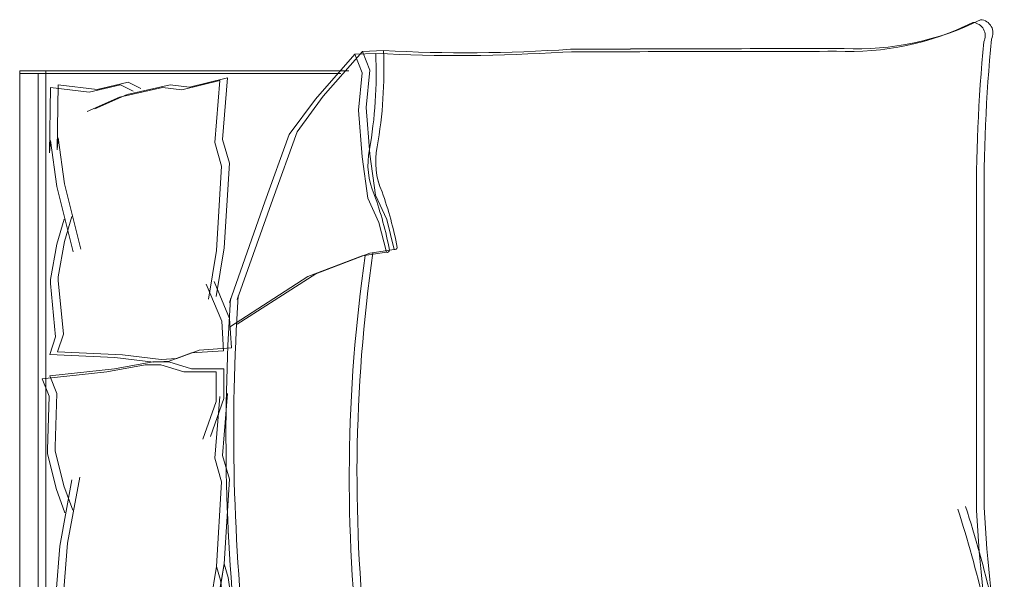
# Model space of a CAD drawing. Units: inches. Extents: x 1885 to 2748, y 783 to 2421.
# Tile 35 of 117: x 2014 to 2095, y 1443 to 1490. Entities that reach past the tile are written whole.
import ezdxf

# ---------------------------------------------------------------- set-up
doc = ezdxf.new("R2010")
doc.units = ezdxf.units.IN
doc.layers.add('A-FURN', color=8, linetype='Continuous', lineweight=13)

# ---------------------------------------------------------------- blocks, each defined once
blk = doc.blocks.new('BED-DOUBLE')
for p, q in [((28.389, 53.095), (25.139, 49.389)), ((28.389, 53.094), (25.139, 49.389)), ((30.133, 53.174), (28.389, 53.095, 3.871)), ((30.133, 53.174), (28.389, 53.094, 3.871)), ((29.008, 51.558), (28.389, 53.095)), ((29.008, 51.557), (28.389, 53.094)), ((27.749, 52.866), (24.499, 49.161)), ((27.75, 52.866), (24.499, 49.161)), ((29.494, 52.946), (27.749, 52.866, 3.871)), ((28.369, 51.329), (27.749, 52.866)), ((29.494, 52.945), (27.75, 52.866, 3.871)), ((28.369, 51.329), (27.75, 52.866)), ((0.004, 51.493), (0.643, 51.492)), ((0.004, 3.474), (0.004, 51.493)), ((0.643, 51.493), (27.253, 51.493)), ((0.643, 51.492), (27.253, 51.492)), ((2.177, 3.702), (2.177, 51.493)), ((2.177, 3.702), (2.177, 51.492)), ((28.698, 48.46), (29.008, 51.558)), ((28.698, 48.46), (29.008, 51.557)), ((0.004, 51.264), (26.614, 51.264)), ((0.004, 51.264), (26.614, 51.264)), ((1.537, 3.474), (1.537, 51.264)), ((1.537, 3.474), (1.537, 51.264)), ((16.576, 50.697), (13.438, 49.922)), ((16.576, 50.697), (13.438, 49.921)), ((17.216, 50.925), (14.077, 50.15)), ((17.216, 50.925), (14.077, 50.15)), ((16.173, 45.565), (16.576, 50.697)), ((16.173, 45.565), (16.576, 50.697)), ((16.812, 45.794), (17.216, 50.925)), ((16.812, 45.793), (17.216, 50.925)), ((28.059, 48.232), (28.369, 51.329)), ((28.059, 48.231), (28.369, 51.329)), ((2.561, 50.111), (2.464, 44.708)), ((2.561, 50.11), (2.464, 44.708)), ((2.561, 50.111), (5.771, 49.732)), ((2.561, 50.11), (5.771, 49.732)), ((3.2, 50.339), (3.103, 44.937)), ((3.2, 50.339), (3.103, 44.936)), ((3.2, 50.339), (6.411, 49.96)), ((3.2, 50.339), (6.411, 49.96)), ((5.771, 49.732), (8.342, 50.327)), ((5.771, 49.732), (8.342, 50.327)), ((6.411, 49.96), (8.981, 50.556)), ((6.411, 49.96), (8.981, 50.555)), ((11.832, 50.111), (8.261, 49.308)), ((11.832, 50.111), (8.261, 49.308)), ((8.342, 50.327), (9.388, 49.813)), ((8.342, 50.327), (9.388, 49.813)), ((12.472, 50.339), (8.9, 49.537)), ((12.472, 50.339), (8.9, 49.536)), ((8.981, 50.556), (10.027, 50.042)), ((8.981, 50.555), (10.027, 50.041)), ((13.438, 49.922), (11.832, 50.111)), ((13.438, 49.921), (11.832, 50.111)), ((14.077, 50.15), (12.472, 50.339)), ((14.077, 50.15), (12.472, 50.339)), ((8.261, 49.308), (5.582, 48.127)), ((8.261, 49.308), (5.582, 48.127)), ((8.9, 49.537), (6.221, 48.355)), ((8.9, 49.536), (6.221, 48.355)), ((24.499, 49.161), (22.332, 46.218)), ((24.499, 49.161), (22.332, 46.218)), ((25.139, 49.389), (22.972, 46.447)), ((25.139, 49.389), (22.972, 46.447)), ((28.369, 44.36), (28.059, 48.232)), ((28.369, 44.36), (28.059, 48.231)), ((29.008, 44.588), (28.698, 48.46)), ((29.008, 44.588), (28.698, 48.46)), ((2.464, 44.708), (2.546, 45.711)), ((2.464, 44.708), (2.546, 45.711)), ((2.546, 45.711), (3.073, 41.913)), ((2.546, 45.711), (3.073, 41.913)), ((3.103, 44.937), (3.185, 45.939)), ((3.103, 44.936), (3.185, 45.939)), ((3.185, 45.939), (3.712, 42.141)), ((3.185, 45.939), (3.712, 42.141)), ((17.369, 43.833), (16.812, 45.794)), ((17.369, 43.833), (16.812, 45.793)), ((22.332, 46.218), (20.32, 40.643)), ((22.332, 46.218), (20.32, 40.643)), ((22.972, 46.447), (20.96, 40.871)), ((22.972, 46.447), (20.96, 40.871)), ((16.73, 43.605), (16.173, 45.565)), ((16.73, 43.605), (16.173, 45.565)), ((28.833, 40.953), (28.369, 44.36)), ((28.833, 40.952), (28.369, 44.36)), ((29.472, 41.181), (29.008, 44.588)), ((29.472, 41.181), (29.008, 44.588)), ((16.299, 36.595), (16.73, 43.605)), ((16.299, 36.595), (16.73, 43.605)), ((16.938, 36.823), (17.369, 43.833)), ((16.938, 36.823), (17.369, 43.833)), ((3.073, 41.913), (4.426, 36.494)), ((3.073, 41.913), (4.426, 36.493)), ((3.712, 42.141), (5.065, 36.722)), ((3.712, 42.141), (5.065, 36.722)), ((20.96, 40.871), (18.026, 32.533)), ((20.96, 40.871), (18.026, 32.533)), ((29.762, 38.939), (28.833, 40.953)), ((29.762, 38.939), (28.833, 40.952)), ((30.401, 39.168), (29.472, 41.181)), ((30.401, 39.167), (29.472, 41.181)), ((20.32, 40.643), (17.387, 32.305)), ((20.32, 40.643), (17.387, 32.305)), ((3.677, 39.199), (3.082, 37.134)), ((3.677, 39.199), (3.082, 37.134)), ((4.317, 39.427), (3.721, 37.362)), ((4.317, 39.427), (3.721, 37.362)), ((31.02, 36.69), (30.401, 39.168)), ((31.02, 36.689), (30.401, 39.167)), ((79.249, 15.062), (79.249, 39.676)), ((79.249, 15.062), (79.249, 39.676)), ((79.888, 15.29), (79.888, 39.904)), ((79.888, 15.29), (79.888, 39.904)), ((30.381, 36.461), (29.762, 38.939)), ((30.381, 36.461), (29.762, 38.939)), ((3.082, 37.134), (2.541, 34.203)), ((3.082, 37.134), (2.541, 34.203)), ((3.721, 37.362), (3.18, 34.432)), ((3.721, 37.362), (3.18, 34.431)), ((16.271, 32.791), (16.938, 36.823)), ((16.272, 32.791), (16.938, 36.823)), ((15.632, 32.563), (16.299, 36.595)), ((15.632, 32.563), (16.299, 36.595)), ((23.88, 34.448), (28.369, 36.152)), ((23.88, 34.448), (28.369, 36.151)), ((24.519, 34.676), (29.008, 36.38)), ((24.519, 34.676), (29.008, 36.38)), ((28.369, 36.152), (30.381, 36.461)), ((28.369, 36.151), (30.381, 36.461)), ((29.008, 36.38), (31.02, 36.69)), ((29.008, 36.38), (31.02, 36.689)), ((3.18, 34.432), (3.2, 34.111)), ((3.18, 34.431), (3.2, 34.11)), ((17.387, 30.258), (23.88, 34.448)), ((17.387, 30.258), (23.88, 34.448)), ((18.026, 30.486), (24.519, 34.676)), ((18.026, 30.486), (24.519, 34.676)), ((2.541, 34.203), (2.561, 33.882)), ((2.541, 34.203), (2.561, 33.882)), ((2.561, 33.882), (2.982, 29.454)), ((2.561, 33.882), (2.982, 29.454)), ((3.2, 34.111), (3.622, 29.683)), ((3.2, 34.11), (3.622, 29.683)), ((16.743, 30.749), (15.458, 33.819)), ((16.743, 30.749), (15.458, 33.819)), ((17.382, 30.977), (16.097, 34.048)), ((17.382, 30.977), (16.097, 34.048)), ((16.896, 28.296), (16.743, 30.749)), ((16.896, 28.296), (16.743, 30.749)), ((17.536, 28.525), (17.382, 30.977)), ((17.536, 28.524), (17.382, 30.977)), ((2.982, 29.454), (2.495, 27.976)), ((2.982, 29.454), (2.495, 27.975)), ((3.622, 29.683), (3.135, 28.204)), ((3.622, 29.683), (3.135, 28.204)), ((2.495, 27.976), (7.871, 27.732)), ((2.495, 27.975), (7.871, 27.732)), ((3.135, 28.204), (8.51, 27.961)), ((3.135, 28.204), (8.51, 27.96)), ((7.871, 27.732), (11.082, 27.354)), ((7.871, 27.732), (11.082, 27.353)), ((8.51, 27.961), (11.721, 27.582)), ((8.51, 27.96), (11.721, 27.582)), ((12.38, 27.435), (14.22, 28.129)), ((12.38, 27.434), (14.22, 28.129)), ((13.02, 27.663), (14.86, 28.357)), ((13.02, 27.663), (14.86, 28.357)), ((14.22, 28.129), (16.896, 28.296)), ((14.22, 28.129), (16.896, 28.296)), ((14.86, 28.357), (17.536, 28.525)), ((14.86, 28.357), (17.536, 28.524)), ((7.224, 26.56), (10.404, 27.138)), ((7.224, 26.559), (10.405, 27.137)), ((7.863, 26.788), (11.044, 27.366)), ((7.863, 26.788), (11.044, 27.366)), ((10.404, 27.138), (11.706, 27.138)), ((10.405, 27.137), (11.706, 27.137)), ((11.044, 27.366), (12.345, 27.366)), ((11.044, 27.366), (12.345, 27.366)), ((11.082, 27.354), (12.38, 27.435)), ((11.082, 27.353), (12.38, 27.434)), ((11.706, 27.138), (13.585, 26.56)), ((11.706, 27.137), (13.585, 26.559)), ((11.721, 27.582), (13.02, 27.663)), ((11.721, 27.582), (13.02, 27.663)), ((12.345, 27.366), (14.225, 26.788)), ((12.345, 27.366), (14.225, 26.788)), ((1.874, 25.981), (7.224, 26.56)), ((1.874, 25.981), (7.224, 26.559)), ((2.513, 26.21), (7.863, 26.788)), ((2.513, 26.209), (7.863, 26.788)), ((3.091, 24.764), (2.513, 26.21)), ((3.091, 24.764), (2.513, 26.209)), ((13.585, 26.56), (16.267, 26.56)), ((13.585, 26.559), (16.267, 26.559)), ((14.225, 26.788), (16.906, 26.788)), ((14.225, 26.788), (16.906, 26.788)), ((16.267, 26.56), (16.267, 24.102)), ((16.267, 26.559), (16.267, 24.102)), ((16.906, 26.788), (16.906, 24.33)), ((16.906, 26.788), (16.906, 24.33)), ((2.452, 24.536), (1.874, 25.981)), ((2.452, 24.535), (1.874, 25.981)), ((2.308, 20.09), (2.452, 24.536)), ((2.308, 20.09), (2.452, 24.535)), ((2.947, 20.319), (3.091, 24.764)), ((2.947, 20.318), (3.091, 24.764)), ((16.173, 19.383), (16.576, 24.515)), ((16.173, 19.382), (16.576, 24.514)), ((16.812, 19.611), (17.216, 24.743)), ((16.812, 19.611), (17.216, 24.743)), ((16.267, 24.102), (15.176, 20.957)), ((16.267, 24.102), (15.176, 20.957)), ((16.906, 24.33), (15.815, 21.186)), ((16.906, 24.33), (15.815, 21.186)), ((2.308, 19.769), (2.308, 20.09)), ((2.308, 19.768), (2.308, 20.09)), ((3.031, 16.877), (2.308, 19.769)), ((3.031, 16.877), (2.308, 19.768)), ((2.947, 19.997), (2.947, 20.319)), ((2.947, 19.997), (2.947, 20.318)), ((3.67, 17.106), (2.947, 19.997)), ((3.67, 17.105), (2.947, 19.997)), ((17.369, 17.651), (16.812, 19.611)), ((17.369, 17.65), (16.812, 19.611)), ((16.73, 17.422), (16.173, 19.383)), ((16.73, 17.422), (16.173, 19.382)), ((3.32, 12.107), (4.332, 17.6)), ((3.32, 12.107), (4.332, 17.6)), ((3.959, 12.335), (4.971, 17.829)), ((3.959, 12.335), (4.971, 17.828)), ((16.299, 10.412), (16.73, 17.422)), ((16.299, 10.412), (16.73, 17.422)), ((16.938, 10.641), (17.369, 17.651)), ((16.938, 10.64), (17.369, 17.65)), ((3.753, 14.854), (3.031, 16.877)), ((3.753, 14.853), (3.031, 16.877)), ((4.393, 15.082), (3.67, 17.106)), ((4.393, 15.082), (3.67, 17.105)), ((3.67, 8.512), (3.959, 12.335)), ((3.67, 8.512), (3.959, 12.335)), ((3.031, 8.284), (3.32, 12.107)), ((3.031, 8.283), (3.32, 12.107)), ((16.271, 6.609), (16.938, 10.641)), ((16.272, 6.609), (16.938, 10.64)), ((16.938, 10.641), (17.261, 9.508)), ((16.938, 10.64), (17.261, 9.507)), ((15.632, 6.38), (16.299, 10.412)), ((15.632, 6.38), (16.299, 10.412)), ((16.299, 10.412), (16.622, 9.279)), ((16.299, 10.412), (16.622, 9.279)), ((16.622, 9.279), (17.345, 4.183)), ((16.622, 9.279), (17.345, 4.182)), ((17.261, 9.508), (17.984, 4.411)), ((17.261, 9.507), (17.984, 4.411)), ((3.012, 8.178), (3.031, 8.284)), ((3.012, 8.178), (3.031, 8.283)), ((3.342, 3.897), (3.012, 8.178)), ((3.342, 3.897), (3.012, 8.178)), ((3.652, 8.407), (3.67, 8.512)), ((3.652, 8.406), (3.67, 8.512)), ((3.981, 4.126), (3.652, 8.407)), ((3.981, 4.125), (3.652, 8.406)), ((8.959, 5.05), (6.211, 6.062)), ((8.959, 5.05), (6.211, 6.061)), ((9.598, 5.278), (6.851, 6.29)), ((9.598, 5.278), (6.851, 6.29)), ((12.573, 4.472), (8.959, 5.05)), ((12.573, 4.471), (8.959, 5.05)), ((13.213, 4.7), (9.598, 5.278)), ((13.213, 4.7), (9.598, 5.278)), ((14.803, 4.989), (13.213, 4.7)), ((14.803, 4.989), (13.213, 4.7)), ((17.984, 4.411), (14.803, 4.989)), ((17.984, 4.411), (14.803, 4.989)), ((3.32, 3.893), (6.501, 4.472)), ((3.32, 3.893), (6.501, 4.471)), ((3.959, 4.122), (7.14, 4.7)), ((3.959, 4.121), (7.14, 4.7)), ((6.501, 4.472), (9.103, 4.038)), ((6.501, 4.471), (9.103, 4.038)), ((7.14, 4.7), (9.743, 4.266)), ((7.14, 4.7), (9.743, 4.266)), ((9.103, 4.038), (10.115, 4.616)), ((9.103, 4.038), (10.115, 4.616)), ((9.743, 4.266), (10.755, 4.845)), ((9.743, 4.266), (10.755, 4.844)), ((14.164, 4.761), (12.573, 4.472)), ((14.164, 4.76), (12.573, 4.471)), ((17.345, 4.183), (14.164, 4.761)), ((17.345, 4.182), (14.164, 4.76)), ((18.114, 3.474), (0.004, 3.474)), ((18.114, 3.474), (0.004, 3.474)), ((18.753, 3.702), (0.643, 3.702)), ((18.753, 3.702), (0.643, 3.702))]:
    blk.add_line(p, q)
for centre, radius, start, end in [((68.67, 76.156), 23.065, 267.47136, 296.46809), ((68.67, 76.156), 23.065, 267.47136, 296.46809), ((69.309, 76.384), 23.065, 267.47136, 296.46809), ((69.309, 76.384), 23.065, 267.47136, 296.46809), ((78.874, 54.409), 1.102, 332.65876, 86.02002), ((78.874, 54.408), 1.102, 332.65876, 86.02002), ((79.513, 54.637), 1.102, 332.65876, 86.02002), ((79.513, 54.637), 1.102, 332.65876, 86.02002), ((212.28, 41.151), 133.04, 174.4998, 180.63509), ((212.28, 41.15), 133.04, 174.4998, 180.63509), ((212.92, 41.379), 133.04, 174.4998, 180.63509), ((212.92, 41.379), 133.04, 174.4998, 180.63509), ((36.319, 182.265), 129.499, 266.97912, 273.83645), ((36.319, 182.264), 129.499, 266.97912, 273.83645), ((-6.013, 51.554), 36.183, 349.87628, 2.56571), ((-6.013, 51.554), 36.183, 349.87628, 2.56571), ((36.958, 182.493), 129.499, 266.97912, 273.83645), ((36.958, 182.493), 129.499, 266.97912, 273.83645), ((67.825, -4508.745), 4561.858, 90.002168, 90.286887), ((67.825, -4508.745), 4561.858, 90.002168, 90.286887), ((68.464, -4508.516), 4561.858, 90.002168, 90.286887), ((68.464, -4508.517), 4561.858, 90.002168, 90.286887), ((-6.653, 51.326), 36.183, 349.87628, 2.56571), ((-6.653, 51.326), 36.183, 349.87628, 2.56571), ((35.07, 43.742), 6.224, 168.6608, 203.73842), ((35.07, 43.742), 6.224, 168.6608, 203.73842), ((35.709, 43.971), 6.224, 168.6608, 203.73842), ((35.709, 43.97), 6.224, 168.6608, 203.73842), ((1.486, 31.152), 29.654, 10.66171, 19.88058), ((1.486, 31.152), 29.654, 10.66171, 19.88058), ((2.125, 31.381), 29.654, 10.66171, 19.88058), ((2.125, 31.381), 29.654, 10.66171, 19.88058), ((31.082, 36.863), 0.185, 250.24637, 1.13765), ((31.082, 36.863), 0.185, 250.24637, 1.13765), ((156.32, 17.754), 129.02, 171.78449, 186.90062), ((156.32, 17.754), 129.02, 171.78449, 186.90062), ((156.959, 17.983), 129.02, 171.78449, 186.90062), ((156.959, 17.983), 129.02, 171.78449, 186.90062), ((30.443, 36.635), 0.185, 250.24637, 1.13765), ((30.443, 36.635), 0.185, 250.24637, 1.13765), ((182.695, 21.586), 164.969, 176.08655, 186.78213), ((182.695, 21.586), 164.969, 176.08655, 186.78213), ((182.056, 21.358), 164.969, 176.08655, 186.78213), ((182.056, 21.357), 164.969, 176.08655, 186.78213), ((-23.708, -17.223), 106.459, 13.38322, 17.70533), ((-23.708, -17.223), 106.459, 13.38322, 17.70533), ((-23.069, -16.995), 106.459, 13.38322, 17.70533), ((-23.069, -16.995), 106.459, 13.38322, 17.70533), ((200.841, 21.425), 121.759, 182.99578, 189.40907), ((200.841, 21.425), 121.759, 182.99578, 189.40907), ((201.48, 21.654), 121.759, 182.99578, 189.40907), ((201.48, 21.654), 121.759, 182.99578, 189.40907), ((20.739, 85.389), 83.306, 268.72178, 275.60397), ((20.739, 85.389), 83.306, 268.72178, 275.60397), ((31.177, -167.309), 170.11, 88.4762, 91.00819), ((31.177, -167.309), 170.11, 88.4762, 91.00819), ((31.817, -167.08), 170.11, 88.4762, 91.00819), ((31.817, -167.081), 170.11, 88.4762, 91.00819), ((50.617, 484.821), 482.31, 268.22771, 271.71854), ((50.617, 484.821), 482.31, 268.22771, 271.71854), ((51.257, 485.049), 482.31, 268.22771, 271.71854), ((51.257, 485.049), 482.31, 268.22771, 271.71854), ((64.519, -26.901), 29.634, 76.06484, 88.91125), ((64.519, -26.901), 29.634, 76.06484, 88.91125), ((65.158, -26.672), 29.634, 76.06484, 88.91125), ((65.158, -26.673), 29.634, 76.06484, 88.91125), ((20.1, 85.16), 83.306, 268.72178, 275.60397), ((20.1, 85.16), 83.306, 268.72178, 275.60397), ((70.279, -21.661), 23.562, 67.97508, 86.652), ((70.279, -21.661), 23.562, 67.97508, 86.652), ((70.919, -21.432), 23.562, 67.97508, 86.652), ((70.919, -21.433), 23.562, 67.97508, 86.652), ((80.361, 1.315), 1.089, 236.17358, 23.47814), ((80.361, 1.314), 1.089, 236.17358, 23.47814), ((79.721, 1.086), 1.089, 236.17358, 23.47814), ((79.721, 1.086), 1.089, 236.17358, 23.47814)]:
    blk.add_arc(centre, radius, start, end)

msp = doc.modelspace()

# ---------------------------------------------------------------- block references
at = {"layer": 'A-FURN'}
msp.add_blockref('BED-DOUBLE', (2013.681, 1434.14), dxfattribs=at)

doc.saveas('drawing.dxf')
